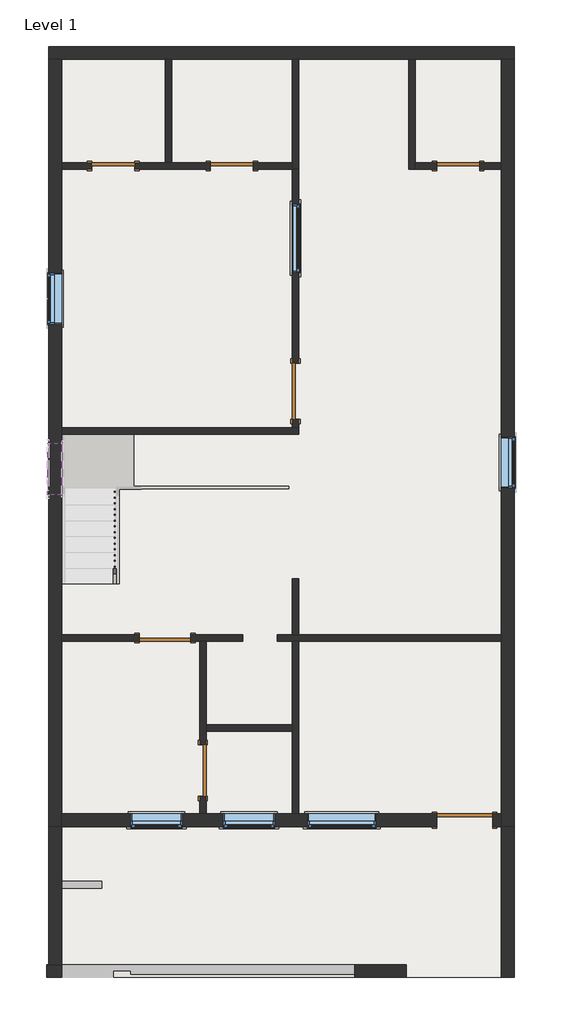
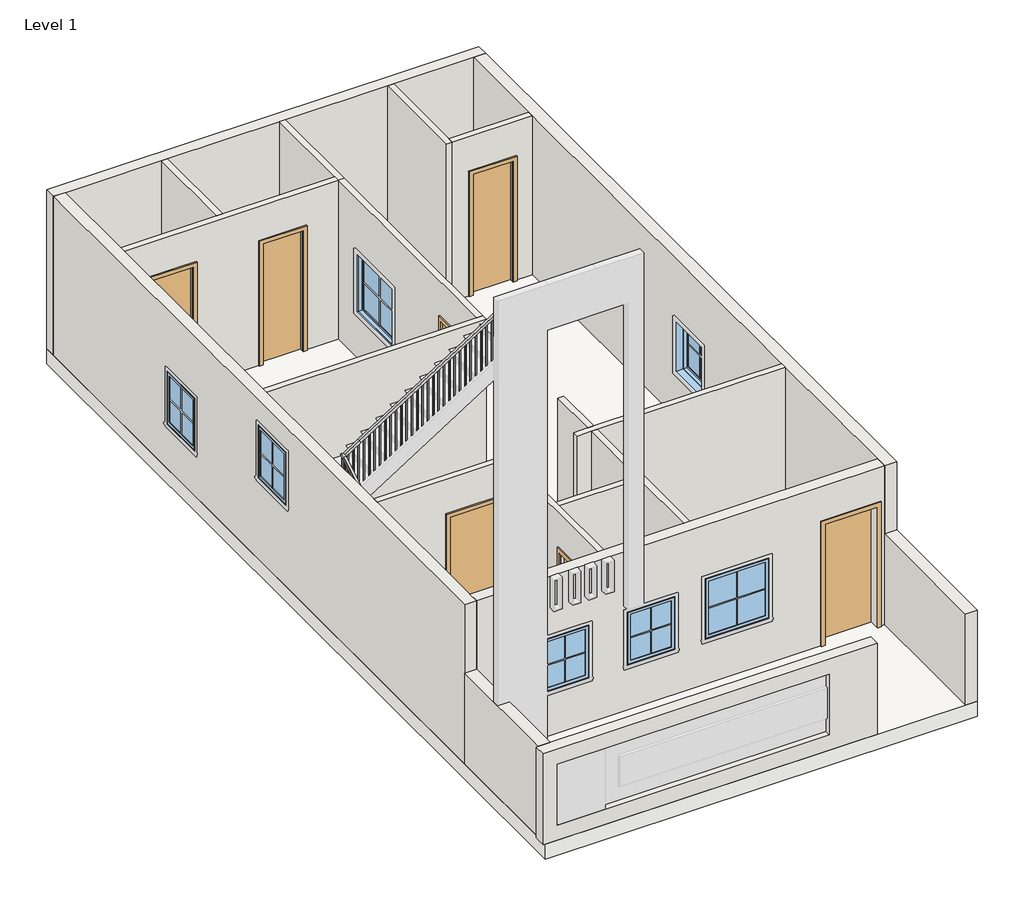
# One storey, part 1 of 2: 19 walls, 7 doors, 7 windows, 1 railing, 1 slab.
# Revit data of these elements (continued)
# Element 34 (IfcWindow, "Window-Casement-Single_Left : W3 3' X 3'6\"") (continued)
#   Materials on its faces: "Wood - Stained", "Glass", "Clad - White"
# Element 35 (IfcWindow, "Window-Casement-Single_Left : W3 3' X 3'6\"")
#   Mark = "14"
#   Window Inset = 0' - 0"
#   Interior Wall Closure = 0' - 2 1/4"
#   Frame Extension = 0' - 0 1/4"
#   Exterior Wall Closure = 0' - 1 1/4"
#   Interior Trim Visibility = yes
#   Exterior Trim Visibility = yes
#   Phase Created = New Construction
#   Materials on its faces: "Wood - Stained", "Glass", "Clad - White"
# Materials
#   "Door - Panel": class "Wood", colour RGB 210 159 95, transparency 0, Cost = 0
#   "Door - Frame": colour RGB 118 70 51, transparency 0, Cost = 0
#   "Wood - Stained": class "Wood", colour RGB 224 178 126, transparency 0, Cost = 0
#   "Glass": class "Glass", colour RGB 0 128 192, transparency 0.75, Description = "Soda Lime Glass", Cost = 0
#   "Clad - White": class "Wood", colour RGB 242 242 238, transparency 0, Cost = 0
#   "Default Floor": colour RGB 128 128 128, transparency 0, Cost = 0
#   "Default Wall": colour RGB 128 128 128, transparency 0, Cost = 0
